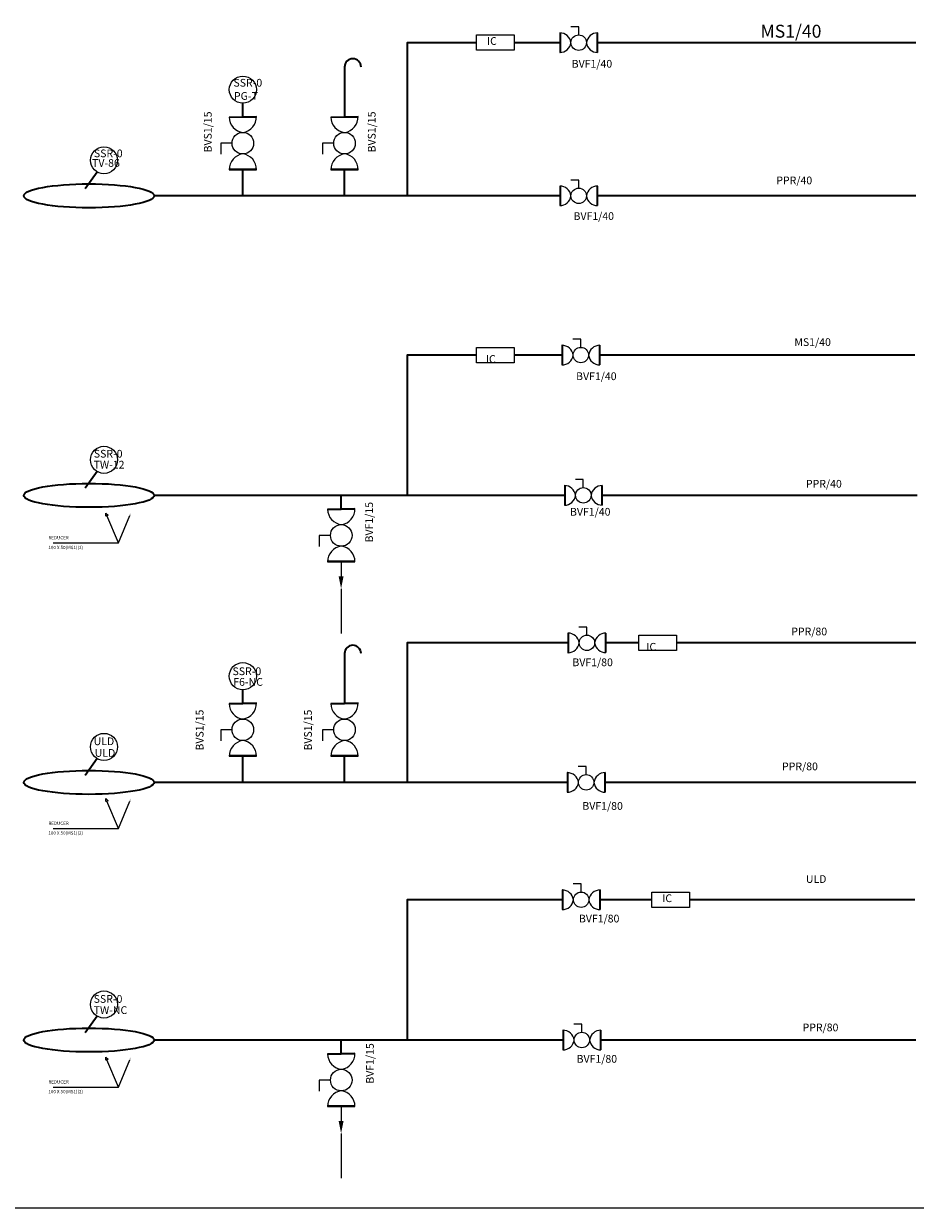
# Model space of a CAD drawing. Units: millimetres. Extents: x 353872 to 441597, y 126154 to 187356.
# Tile 26 of 28: x 415084 to 426416, y 157105 to 172151. Entities that reach past the tile are written whole.
import ezdxf

# ---------------------------------------------------------------- set-up
doc = ezdxf.new("R2010")
doc.units = ezdxf.units.MM
doc.linetypes.add('ACAD_ISO02W100', pattern=[15, 12, -3])
doc.layers.add('AC-UINT', color=2, linetype='Continuous')
for name, color, linetype, lineweight in [('P-ANNO-SYMB', 7, 'Continuous', 18), ('P-ANNO-TEXT', 7, 'Continuous', 25), ('P-BNDY', 4, 'ACAD_ISO02W100', 25), ('P-INST', 6, 'Continuous', 25), ('P-INST-SIGN', 4, 'Continuous', 18), ('P-PIPE', 3, 'Continuous', 35), ('P-PIPE-FITT', 6, 'Continuous', 25), ('P-SYMB-PATT', 8, 'Continuous', 13), ('P-VALV', 2, 'Continuous', 25)]:
    doc.layers.add(name, color=color, linetype=linetype, lineweight=lineweight)
doc.styles.get("Standard").update_dxf_attribs({"font": 'arial.ttf'})

# ---------------------------------------------------------------- blocks, each defined once
blk = doc.blocks.new('DFSG')
at = {"layer": 'AC-UINT', "ltscale": 3}
blk.add_line((94.324, -27.16), (94.091, -27.16), dxfattribs=at)
blk.add_solid([(94.091, -27.121), (94.091, -27.199), (93.897, -27.16)], dxfattribs=at)
blk = doc.blocks.new('VALVE-A')
for points in [[(0, 9), (249, 9)], [(0, 6), (249, 6)], [(0, 3), (0, 0), (249, 0), (249, 4)], [(0, 3), (0, 3), (246, 3), (249, 3)]]:
    blk.add_lwpolyline(points)
for centre, radius, start, end in [((143, 1), 143, 97.3612, 180.5798), ((107, 2), 142, 359.2193, 82.8397)]:
    blk.add_arc(centre, radius, start, end)
blk = doc.blocks.new('VALVE-B')
for points in [[(0, 12), (347, 12)], [(0, 8), (347, 8)], [(0, 4), (0, 0), (347, 0), (347, 5)], [(0, 4), (0, 4), (343, 4), (347, 4)]]:
    blk.add_lwpolyline(points)
for centre, radius, start, end in [((199, 2), 199, 97.3612, 180.5798), ((149, 3), 198, 359.2193, 82.8397)]:
    blk.add_arc(centre, radius, start, end)
blk = doc.blocks.new('VALVE-D-INDICATOR')
for points in [[(330, 249), (330, 0)], [(333, 249), (333, 0)], [(336, 249), (339, 249), (339, 0), (335, 0)], [(336, 249), (336, 246), (336, 3), (336, 0)]]:
    blk.add_lwpolyline(points)
blk.add_circle((98, 125), 98)
for centre, radius, start, end in [((338, 106), 143, 89.4202, 172.6388), ((337, 142), 142, 187.1603, 270.7807)]:
    blk.add_arc(centre, radius, start, end)
blk = doc.blocks.new('INST-BUBBLE-PAIR')
blk.add_circle((172, 172), 172)
blk.add_circle((172, 172), 172)

msp = doc.modelspace()

# ---------------------------------------------------------------- hatches: boundary and pattern name
at = {"layer": 'P-SYMB-PATT'}
h = msp.add_hatch(color=256, dxfattribs=at)
h.dxf.hatch_style = 1
h.paths.add_polyline_path([(416128.68, 165936.08), (416128.68, 165897.35), (416156.37, 165908.99)])
h.paths.add_polyline_path([(416420.67, 165908.99), (416448.35, 165897.35), (416448.35, 165936.08)])
h = msp.add_hatch(color=256, dxfattribs=at)
h.dxf.hatch_style = 1
h.paths.add_polyline_path([(416128.68, 162309.01), (416128.68, 162270.28), (416156.37, 162281.92)])
h.paths.add_polyline_path([(416420.67, 162281.92), (416448.35, 162270.28), (416448.35, 162309.01)])
h = msp.add_hatch(color=256, dxfattribs=at)
h.dxf.hatch_style = 1
h.paths.add_polyline_path([(416128.68, 159024.87), (416128.68, 158986.15), (416156.37, 158997.78)])
h.paths.add_polyline_path([(416420.67, 158997.78), (416448.35, 158986.15), (416448.35, 159024.87)])

# ---------------------------------------------------------------- linework, layer by layer
at = {"layer": 'P-ANNO-SYMB'}
for p, q in [((416288.52, 165555.83), (416142.52, 165903.17)), ((416288.52, 161928.76), (416142.52, 162276.1)), ((416288.52, 158644.63), (416142.52, 158991.96))]:
    msp.add_line(p, q, dxfattribs=at)
for points in [[(415457.7, 165555.83), (416288.52, 165555.83), (416434.52, 165903.17)], [(415457.7, 161928.76), (416288.52, 161928.76), (416434.52, 162276.1)], [(415457.7, 158644.63), (416288.52, 158644.63), (416434.52, 158991.96)]]:
    msp.add_lwpolyline(points, dxfattribs=at)
for points in [[(416156.37, 165908.99), (416128.68, 165897.35), (416128.68, 165936.08)], [(416156.37, 162281.92), (416128.68, 162270.28), (416128.68, 162309.01)], [(416156.37, 158997.78), (416128.68, 158986.15), (416128.68, 159024.87)]]:
    msp.add_lwpolyline(points, close=True, dxfattribs=at)
at = {"layer": 'P-BNDY'}
for p, q in [((419118.61, 164974.79), (419118.61, 164404.9)), ((419118.61, 158056.52), (419118.61, 157486.63)), ((436591, 157104.68), (386532.91, 157104.68))]:
    msp.add_line(p, q, dxfattribs=at)
at = {"layer": 'P-INST'}
for centre in [(417869.93, 171314.05), (417869.93, 163863.54)]:
    msp.add_circle(centre, 172.13, dxfattribs=at)
at = {"layer": 'P-INST-SIGN'}
for points in [[(420840.31, 172011.92), (421316.95, 172011.92), (421316.95, 171814.78), (420840.31, 171814.78)], [(420840.31, 168040.33), (421316.95, 168040.33), (421316.95, 167843.19), (420840.31, 167843.19)], [(422902.73, 164385.3), (423379.37, 164385.3), (423379.37, 164188.15), (422902.73, 164188.15)], [(423068.88, 161122.06), (423545.52, 161122.06), (423545.52, 160924.92), (423068.88, 160924.92)]]:
    msp.add_lwpolyline(points, close=True, dxfattribs=at)
at = {"layer": 'P-PIPE'}
for p, q in [((421897.06, 171910.2), (421316.95, 171910.2)), ((426420.76, 171910.2), (422379.04, 171907.06)), ((417869.93, 170969.78), (417869.93, 171141.92)), ((416019.54, 170266.68), (415864.29, 170054.24)), ((417869.95, 169964.7), (417869.95, 170308.97)), ((419162.22, 169964.7), (419162.22, 170308.97)), ((421316.95, 169964.7), (416743.33, 169964.7)), ((421897.06, 169964.7), (421316.95, 169964.7)), ((426420.76, 169964.7), (422379.04, 169964.7)), ((421924.67, 167941.76), (421316.95, 167941.76)), ((426408.13, 167941.76), (422406.66, 167941.76)), ((416019.54, 166462.15), (415864.29, 166249.71)), ((421316.95, 166160.17), (416743.33, 166160.17)), ((419120.8, 165988.03), (419120.8, 166160.17)), ((421955.84, 166160.17), (421316.95, 166160.17)), ((426439.3, 166160.17), (422437.83, 166160.17)), ((422902.73, 164286.73), (422483.58, 164286.73)), ((426420.76, 164286.73), (423379.37, 164286.73)), ((417869.93, 163519.27), (417869.93, 163691.4)), ((416019.54, 162816.17), (415864.29, 162603.73)), ((417869.95, 162514.19), (417869.95, 162858.45)), ((419162.22, 162514.19), (419162.22, 162858.45)), ((421992.45, 162514.19), (416743.33, 162514.19)), ((422902.73, 162514.19), (422474.43, 162514.19)), ((426420.76, 162514.19), (422688.58, 162514.19)), ((423068.88, 161023.49), (422410.14, 161023.49)), ((426411.61, 161023.49), (423545.52, 161023.49)), ((416019.54, 159543.88), (415864.29, 159331.44)), ((421937.3, 159241.9), (416743.33, 159241.9)), ((419120.8, 159069.76), (419120.8, 159241.9)), ((423545.52, 159241.9), (422419.29, 159241.9)), ((426420.76, 159241.9), (423545.52, 159241.9))]:
    msp.add_line(p, q, dxfattribs=at)
for points in [[(420840.31, 171910.2), (419960.17, 171910.2), (419960.17, 169964.7)], [(420840.31, 167941.76), (419960.17, 167941.76), (419960.17, 166160.17)], [(422001.6, 164286.73), (419960.17, 164286.73), (419960.17, 162514.19)], [(421928.15, 161023.49), (419960.17, 161023.49), (419960.17, 159241.9)]]:
    msp.add_lwpolyline(points, dxfattribs=at)
for points in [[(419372.41, 171600.99, 1), (419162.2, 171600.99), (419162.2, 170969.78)], [(419372.41, 164150.47, 1), (419162.2, 164150.47), (419162.2, 163519.27)]]:
    msp.add_lwpolyline(points, format="xyb", dxfattribs=at)
for centre in [(415913.9, 169964.7), (415913.9, 169964.7), (415913.9, 166160.17), (415913.9, 166160.17), (415913.9, 162514.19), (415913.9, 162514.19), (415913.9, 159241.9), (415913.9, 159241.9)]:
    msp.add_ellipse(centre, major_axis=(829.42, 0), ratio=0.18269243, dxfattribs=at)
at = {"layer": 'P-VALV'}
for points in [[(422138.05, 172008.56), (422138.05, 172111.2), (422037.27, 172111.2)], [(417732.62, 170633.34), (417589.32, 170633.34), (417589.32, 170492.64)], [(419024.89, 170633.34), (418881.59, 170633.34), (418881.59, 170492.64)], [(422138.05, 170063.06), (422138.05, 170165.7), (422037.27, 170165.7)], [(422165.66, 168040.12), (422165.66, 168142.77), (422064.89, 168142.77)], [(422196.83, 166258.52), (422196.83, 166361.17), (422096.06, 166361.17)], [(418983.49, 165651.59), (418840.19, 165651.59), (418840.19, 165510.9)], [(422242.59, 164385.08), (422242.59, 164487.73), (422141.81, 164487.73)], [(417732.62, 163182.82), (417589.32, 163182.82), (417589.32, 163042.13)], [(419024.89, 163182.82), (418881.59, 163182.82), (418881.59, 163042.13)], [(422233.44, 162612.54), (422233.44, 162715.19), (422132.66, 162715.19)], [(422169.15, 161121.85), (422169.15, 161224.49), (422068.37, 161224.49)], [(422178.3, 159340.25), (422178.3, 159442.9), (422077.52, 159442.9)], [(418983.49, 158733.32), (418840.19, 158733.32), (418840.19, 158592.62)]]:
    msp.add_lwpolyline(points, dxfattribs=at)
for centre in [(417869.47, 170633.34), (419161.74, 170633.34), (419120.34, 165651.59), (417869.47, 163182.82), (419161.74, 163182.82), (419120.34, 158733.32)]:
    msp.add_circle(centre, 136.85, dxfattribs=at)

# ---------------------------------------------------------------- block references
at = {"layer": 'P-INST'}
for p in [(415932.83, 170243.99), (415932.83, 166439.46), (415932.83, 162793.48), (415932.83, 159521.19)]:
    msp.add_blockref('INST-BUBBLE-PAIR', p, dxfattribs=at)
at = {"layer": 'P-PIPE-FITT', "xscale": 805.9348046081378, "yscale": 805.9348046081378, "zscale": 805.9348046081378, "rotation": 89.99999999999991}
for p in [(397229.57, 89300.32), (397229.57, 82382.04)]:
    msp.add_blockref('DFSG', p, dxfattribs=at)
at = {"layer": 'P-VALV'}
for name, p, rotation in [('VALVE-A', (421897.06, 172034.57), 269.999999999922), ('VALVE-B', (418042.8, 170973.73), 181.3019170021908), ('VALVE-B', (419335.08, 170973.73), 181.3019170021883), ('VALVE-A', (421897.06, 170089.07), 269.999999999922), ('VALVE-A', (421924.67, 168066.14), 269.9999999999745), ('VALVE-A', (421955.84, 166284.54), 269.9999999998978), ('VALVE-B', (419293.67, 165991.98), 181.3019170022028), ('VALVE-A', (422001.6, 164411.1), 269.9999999999259), ('VALVE-B', (418042.8, 163523.21), 181.3019170022003), ('VALVE-B', (419335.08, 163523.21), 181.3019170022028), ('VALVE-A', (421992.45, 162638.56), 269.9999999999745), ('VALVE-A', (421928.15, 161147.86), 269.9999999999783), ('VALVE-A', (421937.3, 159366.27), 269.9999999999521), ('VALVE-B', (419293.67, 159073.7), 181.3019170021841)]:
    msp.add_blockref(name, p, dxfattribs=dict(at, rotation=rotation))
for name, p in [('VALVE-D-INDICATOR', (422040.02, 171785.82)), ('VALVE-B', (417696.3, 170296.89)), ('VALVE-B', (418988.57, 170296.89)), ('VALVE-D-INDICATOR', (422040.02, 169840.32)), ('VALVE-D-INDICATOR', (422067.64, 167817.38)), ('VALVE-D-INDICATOR', (422098.81, 166035.79)), ('VALVE-B', (418947.17, 165315.15)), ('VALVE-D-INDICATOR', (422144.56, 164162.34)), ('VALVE-B', (417696.3, 162846.38)), ('VALVE-B', (418988.57, 162846.38)), ('VALVE-D-INDICATOR', (422135.41, 162389.81)), ('VALVE-D-INDICATOR', (422071.12, 160899.11)), ('VALVE-D-INDICATOR', (422080.27, 159117.51)), ('VALVE-B', (418947.17, 158396.87))]:
    msp.add_blockref(name, p, dxfattribs=at)

# ---------------------------------------------------------------- texts
at = {"layer": 'P-ANNO-TEXT'}
for s, height, p in [('MS1/40', 163.985, (424447.84, 171973.72)), ('IC', 98.09, (420973.32, 171882.42)), ('BVF1/40', 98.09, (422049.56, 171593.09)), ('SSR-0', 98.09, (417750.51, 171351.92)), ('PG-T', 98.09, (417756.77, 171184.34)), ('SSR-0', 98.09, (415976.84, 170454.97)), ('TV-86', 98.09, (415954.12, 170333.2)), ('PPR/40', 98.09, (424649.98, 170111.74)), ('BVF1/40', 98.09, (422072.8, 169658.45)), ('MS1/40', 98.09, (424879.22, 168057.8)), ('IC', 98.09, (420958.7, 167843.19)), ('BVF1/40', 98.09, (422105.41, 167624.27)), ('SSR-0', 98.09, (415975.79, 166640.19)), ('TW-12', 98.09, (415973.03, 166501.03)), ('PPR/40', 98.09, (425026.42, 166258.55)), ('BVF1/40', 98.09, (422027.92, 165902.43)), ('100 X 50(MS1)(2)', 42.1017, (415398.67, 165477.3)), ('REDUCER', 42.102, (415398.67, 165601.11)), ('PPR/80', 98.09, (424839.83, 164381.97)), ('IC', 98.09, (422998.07, 164188.15)), ('BVF1/80', 98.09, (422058.32, 163990.71)), ('SSR-0', 98.09, (417738.72, 163877.24)), ('F6-NC', 98.09, (417748.3, 163741.73)), ('ULD', 98.09, (415973.89, 162987.39)), ('ULD', 98.09, (415987.31, 162839.96)), ('PPR/80', 98.09, (424722.75, 162668.44)), ('BVF1/80', 98.09, (422185.03, 162166.19)), ('REDUCER', 42.102, (415398.67, 161974.04)), ('100 X 50(MS1)(2)', 42.1017, (415398.67, 161850.23)), ('ULD', 98.09, (425025.37, 161237.87)), ('IC', 98.09, (423200.16, 160994.05)), ('BVF1/80', 98.09, (422141.15, 160735.62)), ('SSR-0', 98.09, (415973.89, 159715.1)), ('TW-NC', 98.09, (415973.89, 159572.89)), ('PPR/80', 98.09, (424983.14, 159353.11)), ('BVF1/80', 98.09, (422111.89, 158953.86)), ('100 X 50(MS1)(2)', 42.1017, (415398.67, 158566.1)), ('REDUCER', 42.102, (415398.67, 158689.9))]:
    msp.add_text(s, height=height, dxfattribs=at).set_placement(p)
for s, p in [('BVS1/15', (417473.65, 170516.53)), ('BVS1/15', (419556.77, 170516.53)), ('BVF1/15', (419523.42, 165562.88)), ('BVS1/15', (417369.98, 162919.32)), ('BVS1/15', (418746.82, 162919.32)), ('BVF1/15', (419534.23, 158687.7))]:
    msp.add_text(s, height=98.09, rotation=90, dxfattribs=at).set_placement(p)

doc.saveas('drawing.dxf')
